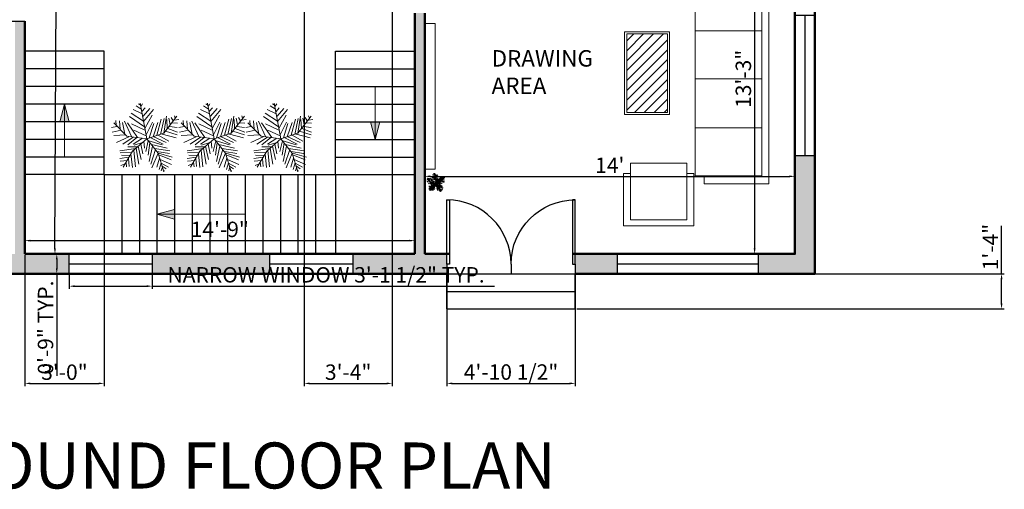
# Model space of a CAD drawing. Units: inches. Extents: x 1647 to 2354, y 1705 to 2321.
# Tile 2 of 4: x 1907 to 2354, y 1705 to 1919. Entities that reach past the tile are written whole.
import ezdxf

# ---------------------------------------------------------------- set-up
doc = ezdxf.new("R2010")
doc.units = ezdxf.units.IN
for name, color, linetype, lineweight in [('A-ANNO-DIMS', 130, 'Continuous', 18), ('A-ANNO-SYMB', 50, 'Continuous', 18), ('A-ANNO-TEXT', 7, 'Continuous', 35), ('A-AREA-IDEN', 7, 'Continuous', 25), ('A-FURN-PATT', 52, 'Continuous', 13), ('A-WALL-PATT', 84, 'Continuous', 13), ('door', 142, 'Continuous', 25), ('fur', 52, 'Continuous', 18), ('stair', 50, 'Continuous', 25), ('tree', 92, 'Continuous', 13), ('wall', 84, 'Continuous', 50), ('window', 242, 'Continuous', 25)]:
    doc.layers.add(name, color=color, linetype=linetype, lineweight=lineweight)
doc.styles.get("Standard").update_dxf_attribs({"font": 'arial.ttf'})
doc.dimstyles.new('ISO-25', dxfattribs={"dimtxt": 7, "dimasz": 2.5, "dimexe": 1.25, "dimexo": 0.625, "dimtad": 1, "dimdec": 0, "dimlunit": 4, "dimtxsty": 'Standard', "dimcen": 2.5, "dimadec": 0, "dimazin": 0, "dimtfac": 1, "dimtdec": 0, "dimtmove": 0, "dimatfit": 3, "dimfxl": 1, "dimarcsym": 0})

# ---------------------------------------------------------------- blocks, each defined once
blk = doc.blocks.new('*U2')
for p, q in [((0, 0), (0, -6)), ((40, 0), (40, -6))]:
    blk.add_line(p, q)
blk.add_lwpolyline([(0, 0), (0, 40), (1.75, 40), (1.75, 0)], close=True)
blk.add_arc((0, 0), 40, 0, 90)
blk = doc.blocks.new('*U6')
for p, q in [((-8.737, 47.138), (-17.069, 52.711)), ((-10.186, 53.64), (-13.084, 55.962)), ((0, 0), (-10.5, 57)), ((-9.099, 51.782), (-6.563, 55.962)), ((-7.65, 43.423), (-2.578, 49.46)), ((-5.839, 35.992), (4.667, 48.067)), ((-3.665, 19.273), (-27.574, 35.527)), ((-5.114, 28.097), (-24.676, 40.636)), ((-7.288, 39.707), (-21.778, 46.673)), ((-5.114, 27.632), (10.463, 46.673)), ((-2.941, 16.486), (8.652, 37.85)), ((16.259, 5.805), (23.142, 31.348)), ((22.055, 7.198), (27.489, 32.277)), ((27, 9), (48, 36)), ((27.127, 9.056), (31.112, 35.992)), ((35.096, 32.741), (37.27, 22.524)), ((38.719, 34.134), (41.979, 28.561)), ((44.153, 36.456), (45.239, 32.741)), ((-47.498, 19.737), (-55.83, 18.344)), ((-31.5, 4.5), (-52.5, 25.5)), ((-48.585, 21.131), (-49.309, 29.026)), ((-43.513, 28.561), (-42.427, 15.558)), ((-38.442, 26.239), (-34.819, 7.663)), ((-35.544, 28.097), (-24.314, 3.947)), ((-14.533, 2.09), (-30.834, 25.31)), ((-24.314, 23.917), (-2.941, 13.7)), ((-1.129, 6.734), (9.014, 26.704)), ((3.942, 1.625), (11.187, 24.381)), ((10.101, 3.483), (17.708, 26.239)), ((31.836, 30.883), (32.561, 16.486)), ((33.285, 16.486), (48.862, 10.913)), ((36.183, 19.737), (48.137, 17.88)), ((40.53, 25.775), (48.862, 24.846)), ((43.791, 29.954), (51.036, 30.883)), ((-40.615, 13.7), (-55.105, 10.913)), ((-33.37, 6.269), (-52.207, 5.34)), ((-28.299, 3.483), (-47.86, -5.805)), ((-21.416, 3.018), (-38.079, -8.128)), ((0, 0), (-31.5, 4.5)), ((-15.982, 2.09), (-30.11, -9.521)), ((0, 0), (-22.5, -19.5)), ((-6.563, 1.161), (-21.416, -8.128)), ((-20.691, 13.7), (-1.129, 4.876)), ((0, 0), (27, 9)), ((0, 0), (18, -22.5)), ((6.478, 1.625), (26.04, -8.592)), ((11.187, 3.483), (30.749, -5.805)), ((18.07, 5.805), (35.096, -3.483)), ((24.229, 7.663), (46.688, 1.625)), ((29.662, 12.307), (48.137, 6.269)), ((-17.431, -15.094), (-42.789, -18.809)), ((-15.257, -12.772), (-30.11, -12.772)), ((-6.563, -5.805), (-19.967, -9.985)), ((-17.069, -15.094), (-12.721, -40.172)), ((-13.446, -11.378), (-8.737, -32.741)), ((-9.461, -8.592), (-6.201, -23.453)), ((-4.752, -3.483), (-3.665, -14.629)), ((2.493, -3.019), (-1.491, -20.202)), ((1.769, -2.555), (24.229, -9.521)), ((5.029, -6.27), (2.131, -25.775)), ((9.014, -11.378), (3.58, -35.992)), ((7.565, -9.056), (32.198, -14.629)), ((12.274, -15.094), (36.907, -18.809)), ((-28.299, -29.026), (-42.789, -31.348)), ((-24.314, -21.596), (-42.427, -22.06)), ((-26.849, -26.24), (-40.253, -25.775)), ((-22.5, -19.5), (-37.5, -45)), ((-29.023, -30.884), (-27.936, -43.887)), ((-25.038, -23.918), (-22.865, -45.281)), ((-20.691, -18.345), (-17.793, -44.352)), ((14.085, -16.951), (6.478, -40.172)), ((18.07, -22.524), (8.289, -45.745)), ((20.244, -30.419), (15.897, -44.816)), ((16.259, -19.738), (36.183, -22.989)), ((18, -22.5), (27, -52.5)), ((18.433, -22.524), (40.53, -29.026)), ((19.157, -25.311), (38.719, -33.206)), ((-30.834, -34.135), (-42.427, -35.528)), ((-34.457, -39.708), (-40.978, -42.494)), ((-32.646, -36.921), (-31.921, -44.352)), ((22.78, -37.85), (19.519, -48.532)), ((21.331, -32.741), (39.081, -40.636)), ((22.78, -38.314), (34.372, -44.816)), ((24.591, -45.745), (23.142, -50.854)), ((24.591, -43.423), (30.749, -47.603)), ((26.764, -49.925), (28.213, -50.854))]:
    blk.add_line(p, q)
blk = doc.blocks.new('*D15')
at = {"layer": 'A-ANNO-DIMS', "color": 0, "lineweight": -2, "transparency": 16777216}
for p, q in [((1909.63, 1812.86), (1909.63, 1819.51)), ((2086.63, 1812.86), (2086.63, 1819.51)), ((1912.13, 1818.26), (2084.13, 1818.26))]:
    blk.add_line(p, q, dxfattribs=at)
at = {"layer": 'A-ANNO-DIMS', "color": 0, "transparency": 16777216}
for points in [[(1912.13, 1818.68), (1912.13, 1817.85), (1909.63, 1818.26)], [(2084.13, 1818.68), (2084.13, 1817.85), (2086.63, 1818.26)]]:
    blk.add_solid(points, dxfattribs=at)
at = {"layer": 'Defpoints', "color": 0, "transparency": 16777216}
for p in [(2086.63, 1818.26), (1909.63, 1812.23), (2086.63, 1812.23)]:
    blk.add_point(p, dxfattribs=at)
at = {"layer": 'A-ANNO-DIMS', "color": 0, "transparency": 16777216, "insert": (1998.13, 1822.46), "char_height": 7, "attachment_point": 5}
blk.add_mtext('14\'-9"', dxfattribs=at)
blk = doc.blocks.new('*D16')
at = {"layer": 'A-ANNO-DIMS', "color": 0, "lineweight": -2, "transparency": 16777216}
for p, q in [((1911.55, 2059.73), (1925.86, 2059.66)), ((1923.34, 1814.66), (1924.6, 2057.16)), ((1910.26, 1812.23), (1924.57, 1812.16))]:
    blk.add_line(p, q, dxfattribs=at)
at = {"layer": 'A-ANNO-DIMS', "color": 0, "transparency": 16777216}
for points in [[(1924.18, 2057.16), (1925.01, 2057.16), (1924.61, 2059.66)], [(1922.92, 1814.66), (1923.75, 1814.66), (1923.32, 1812.16)]]:
    blk.add_solid(points, dxfattribs=at)
at = {"layer": 'Defpoints', "color": 0, "transparency": 16777216}
for p in [(1910.92, 2059.73), (1924.61, 2059.66), (1909.63, 1812.23)]:
    blk.add_point(p, dxfattribs=at)
at = {"layer": 'A-ANNO-DIMS', "color": 0, "transparency": 16777216, "insert": (1919.77, 1935.93), "char_height": 7, "attachment_point": 5, "rotation": 89.702}
blk.add_mtext('20\'-8"', dxfattribs=at)
blk = doc.blocks.new('*D17')
at = {"layer": 'A-ANNO-DIMS', "color": 0, "lineweight": -2, "transparency": 16777216}
for p, q in [((2091.13, 1812.86), (2091.13, 1848.7)), ((2093.63, 1847.45), (2256.63, 1847.45)), ((2259.13, 1812.86), (2259.13, 1848.7))]:
    blk.add_line(p, q, dxfattribs=at)
at = {"layer": 'A-ANNO-DIMS', "color": 0, "transparency": 16777216}
for points in [[(2093.63, 1847.87), (2093.63, 1847.04), (2091.13, 1847.45)], [(2256.63, 1847.87), (2256.63, 1847.04), (2259.13, 1847.45)]]:
    blk.add_solid(points, dxfattribs=at)
at = {"layer": 'Defpoints', "color": 0, "transparency": 16777216}
for p in [(2259.13, 1847.45), (2091.13, 1812.23), (2259.13, 1812.23)]:
    blk.add_point(p, dxfattribs=at)
at = {"layer": 'A-ANNO-DIMS', "color": 0, "transparency": 16777216, "insert": (2175.13, 1851.59), "char_height": 7, "attachment_point": 5}
blk.add_mtext("14'", dxfattribs=at)
blk = doc.blocks.new('*D18')
at = {"layer": 'A-ANNO-DIMS', "color": 0, "lineweight": -2, "transparency": 16777216}
for p, q in [((2258.51, 1971.23), (2239.61, 1971.23)), ((2240.86, 1968.73), (2240.86, 1814.73)), ((2258.51, 1812.23), (2239.61, 1812.23))]:
    blk.add_line(p, q, dxfattribs=at)
at = {"layer": 'A-ANNO-DIMS', "color": 0, "transparency": 16777216}
for points in [[(2240.44, 1968.73), (2241.28, 1968.73), (2240.86, 1971.23)], [(2240.44, 1814.73), (2241.28, 1814.73), (2240.86, 1812.23)]]:
    blk.add_solid(points, dxfattribs=at)
at = {"layer": 'Defpoints', "color": 0, "transparency": 16777216}
for p in [(2259.13, 1971.23), (2240.86, 1812.23), (2259.13, 1812.23)]:
    blk.add_point(p, dxfattribs=at)
at = {"layer": 'A-ANNO-DIMS', "color": 0, "transparency": 16777216, "insert": (2236.66, 1891.73), "char_height": 7, "attachment_point": 5, "rotation": 90}
blk.add_mtext('13\'-3"', dxfattribs=at)
blk = doc.blocks.new('WIN-WIDE-9IN-WALL')
blk.add_line((0, 4.5), (63.83, 4.5))
blk.add_lwpolyline([(0, 9), (63.83, 9), (63.83, 0), (0, 0)], close=True)
blk = doc.blocks.new('WIN-NARROW-9IN-WALL')
blk.add_line((4.5, 0), (4.5, 37.68))
blk.add_lwpolyline([(0, 37.68), (9, 37.68), (9, 0), (0, 0)], close=True)
blk = doc.blocks.new('*D37')
at = {"layer": 'A-ANNO-DIMS', "color": 0, "lineweight": -2, "transparency": 16777216}
for p, q in [((1929.8, 1802.61), (1929.8, 1796.33)), ((1967.48, 1802.61), (1967.48, 1796.33)), ((1932.3, 1797.58), (1964.98, 1797.58)), ((1967.48, 1797.58), (2122.76, 1797.58))]:
    blk.add_line(p, q, dxfattribs=at)
at = {"layer": 'A-ANNO-DIMS', "color": 0, "transparency": 16777216}
for points in [[(1932.3, 1798), (1932.3, 1797.16), (1929.8, 1797.58)], [(1964.98, 1798), (1964.98, 1797.16), (1967.48, 1797.58)]]:
    blk.add_solid(points, dxfattribs=at)
at = {"layer": 'Defpoints', "color": 0, "transparency": 16777216}
for p in [(1929.8, 1803.23), (1967.48, 1803.23), (1967.48, 1797.58)]:
    blk.add_point(p, dxfattribs=at)
at = {"layer": 'A-ANNO-DIMS', "color": 0, "transparency": 16777216, "insert": (2046.37, 1801.83), "char_height": 7, "attachment_point": 5}
blk.add_mtext('NARROW WINDOW 3\'-1 1/2" TYP.', dxfattribs=at)
blk = doc.blocks.new('*D38')
at = {"layer": 'A-ANNO-DIMS', "color": 0, "lineweight": -2, "transparency": 16777216}
for p, q in [((1929.18, 1812.23), (1922.9, 1812.23)), ((1924.15, 1809.73), (1924.15, 1805.73)), ((1929.18, 1803.23), (1922.9, 1803.23)), ((1924.15, 1803.23), (1924.15, 1756.81))]:
    blk.add_line(p, q, dxfattribs=at)
at = {"layer": 'A-ANNO-DIMS', "color": 0, "transparency": 16777216}
for points in [[(1923.74, 1809.73), (1924.57, 1809.73), (1924.15, 1812.23)], [(1923.74, 1805.73), (1924.57, 1805.73), (1924.15, 1803.23)]]:
    blk.add_solid(points, dxfattribs=at)
at = {"layer": 'Defpoints', "color": 0, "transparency": 16777216}
for p in [(1929.8, 1812.23), (1924.15, 1803.23), (1929.8, 1803.23)]:
    blk.add_point(p, dxfattribs=at)
at = {"layer": 'A-ANNO-DIMS', "color": 0, "transparency": 16777216, "insert": (1919.95, 1778.77), "char_height": 7, "attachment_point": 5, "rotation": 90}
blk.add_mtext('0\'-9" TYP.', dxfattribs=at)
blk = doc.blocks.new('*D53')
at = {"layer": 'A-ANNO-DIMS', "color": 0, "lineweight": -2, "transparency": 16777216}
for p, q in [((2101.16, 1802.61), (2101.16, 1752.18)), ((2159.48, 1802.61), (2159.48, 1752.18)), ((2103.66, 1753.43), (2156.98, 1753.43))]:
    blk.add_line(p, q, dxfattribs=at)
at = {"layer": 'A-ANNO-DIMS', "color": 0, "transparency": 16777216}
for points in [[(2103.66, 1753.85), (2103.66, 1753.02), (2101.16, 1753.43)], [(2156.98, 1753.85), (2156.98, 1753.02), (2159.48, 1753.43)]]:
    blk.add_solid(points, dxfattribs=at)
at = {"layer": 'Defpoints', "color": 0, "transparency": 16777216}
for p in [(2101.16, 1803.23), (2159.48, 1803.23), (2159.48, 1753.43)]:
    blk.add_point(p, dxfattribs=at)
at = {"layer": 'A-ANNO-DIMS', "color": 0, "transparency": 16777216, "insert": (2130.32, 1757.68), "char_height": 7, "attachment_point": 5}
blk.add_mtext('4\'-10 1/2"', dxfattribs=at)
blk = doc.blocks.new('*D54')
at = {"layer": 'A-ANNO-DIMS', "color": 0, "lineweight": -2, "transparency": 16777216}
for p, q in [((2352.93, 1803.23), (2352.93, 1824.93)), ((2160.11, 1803.23), (2354.18, 1803.23)), ((2352.93, 1789.73), (2352.93, 1800.73)), ((2160.11, 1787.23), (2354.18, 1787.23))]:
    blk.add_line(p, q, dxfattribs=at)
at = {"layer": 'A-ANNO-DIMS', "color": 0, "transparency": 16777216}
for points in [[(2352.52, 1800.73), (2353.35, 1800.73), (2352.93, 1803.23)], [(2352.52, 1789.73), (2353.35, 1789.73), (2352.93, 1787.23)]]:
    blk.add_solid(points, dxfattribs=at)
at = {"layer": 'Defpoints', "color": 0, "transparency": 16777216}
for p in [(2159.48, 1803.23), (2352.93, 1803.23), (2159.48, 1787.23)]:
    blk.add_point(p, dxfattribs=at)
at = {"layer": 'A-ANNO-DIMS', "color": 0, "transparency": 16777216, "insert": (2348.8, 1815.33), "char_height": 7, "attachment_point": 5, "rotation": 90}
blk.add_mtext('1\'-4"', dxfattribs=at)
blk = doc.blocks.new('*D55')
at = {"layer": 'A-ANNO-DIMS', "color": 0, "lineweight": -2, "transparency": 16777216}
for p, q in [((1909.63, 1811.61), (1909.63, 1752.18)), ((1945.63, 1811.61), (1945.63, 1752.18)), ((1912.13, 1753.43), (1943.13, 1753.43))]:
    blk.add_line(p, q, dxfattribs=at)
at = {"layer": 'A-ANNO-DIMS', "color": 0, "transparency": 16777216}
for points in [[(1912.13, 1753.85), (1912.13, 1753.02), (1909.63, 1753.43)], [(1943.13, 1753.85), (1943.13, 1753.02), (1945.63, 1753.43)]]:
    blk.add_solid(points, dxfattribs=at)
at = {"layer": 'Defpoints', "color": 0, "transparency": 16777216}
for p in [(1909.63, 1812.23), (1945.63, 1812.23), (1945.63, 1753.43)]:
    blk.add_point(p, dxfattribs=at)
at = {"layer": 'A-ANNO-DIMS', "color": 0, "transparency": 16777216, "insert": (1927.63, 1757.63), "char_height": 7, "attachment_point": 5}
blk.add_mtext('3\'-0"', dxfattribs=at)
blk = doc.blocks.new('*D56')
at = {"layer": 'A-ANNO-DIMS', "color": 0, "lineweight": -2, "transparency": 16777216}
for p, q in [((2036.41, 2059.11), (2036.41, 1752.18)), ((2076.41, 2059.11), (2076.41, 1752.18)), ((2038.91, 1753.43), (2073.91, 1753.43))]:
    blk.add_line(p, q, dxfattribs=at)
at = {"layer": 'A-ANNO-DIMS', "color": 0, "transparency": 16777216}
for points in [[(2038.91, 1753.85), (2038.91, 1753.02), (2036.41, 1753.43)], [(2073.91, 1753.85), (2073.91, 1753.02), (2076.41, 1753.43)]]:
    blk.add_solid(points, dxfattribs=at)
at = {"layer": 'Defpoints', "color": 0, "transparency": 16777216}
for p in [(2036.41, 2059.73), (2076.41, 2059.73), (2076.41, 1753.43)]:
    blk.add_point(p, dxfattribs=at)
at = {"layer": 'A-ANNO-DIMS', "color": 0, "transparency": 16777216, "insert": (2056.41, 1757.63), "char_height": 7, "attachment_point": 5}
blk.add_mtext('3\'-4"', dxfattribs=at)

msp = doc.modelspace()

# ---------------------------------------------------------------- hatches: boundary and pattern name
at = {"layer": 'A-ANNO-SYMB'}
h = msp.add_hatch(color=256, dxfattribs=at)
h.dxf.hatch_style = 1
h.paths.add_polyline_path([(1927.63, 1880.23), (1925.48, 1872.23), (1927.63, 1872.23)])
h.paths.add_polyline_path([(1927.63, 1880.23), (1927.63, 1872.23), (1929.78, 1872.23)])
h.paths.add_polyline_path([(1977.63, 1830.23), (1969.63, 1830.23), (1977.63, 1828.08)])
h.paths.add_polyline_path([(1977.63, 1832.38), (1969.63, 1830.23), (1977.63, 1830.23)])
h.paths.add_polyline_path([(2068.63, 1872.23), (2066.48, 1872.23), (2068.63, 1864.23)])
h.paths.add_polyline_path([(2070.78, 1872.23), (2068.63, 1872.23), (2068.63, 1864.23)])
at = {"layer": 'A-FURN-PATT'}
h = msp.add_hatch(dxfattribs=at)
h.set_pattern_fill('ANSI31', color=256)
h.paths.add_polyline_path([(2201.3, 1912.1), (2182.82, 1912.1), (2182.82, 1876.48), (2201.3, 1876.48)])
at = {"layer": 'A-WALL-PATT'}
h = msp.add_hatch(color=256, dxfattribs=at)
h.dxf.hatch_style = 1
h.paths.add_polyline_path([(1737.13, 2214.23), (1778.6, 2214.23), (1778.6, 2223.23), (1728.13, 2223.23), (1728.13, 2080.92), (1737.13, 2080.92)])
h.paths.add_polyline_path([(1785.23, 1812.23), (1737.13, 1812.23), (1737.13, 1856.57), (1728.13, 1856.57), (1728.13, 1803.23), (1785.23, 1803.23)])
h.paths.add_polyline_path([(2020.88, 1812.23), (1967.48, 1812.23), (1967.48, 1803.23), (2020.88, 1803.23)])
h.paths.add_polyline_path([(2101.16, 1807.61), (2101.16, 1812.23), (2091.13, 1812.23), (2091.13, 1921.55), (2086.63, 1921.55), (2086.63, 1812.23), (2058.56, 1812.23), (2058.56, 1803.23), (2101.16, 1803.23)])
h.paths.add_polyline_path([(1929.8, 1812.23), (1909.63, 1812.23), (1909.63, 1848.23), (1909.63, 1917.89), (1905.13, 1917.89), (1905.13, 1812.23), (1882.72, 1812.23), (1849.06, 1812.23), (1849.06, 1803.23), (1929.8, 1803.23)])
h.paths.add_polyline_path([(2178.59, 1812.23), (2159.48, 1812.23), (2159.48, 1807.61), (2159.48, 1803.23), (2178.59, 1803.23)])
h.paths.add_polyline_path([(2268.13, 1856.83), (2259.13, 1856.83), (2259.13, 1815.23), (2259.13, 1812.23), (2242.42, 1812.23), (2242.42, 1803.23), (2268.13, 1803.23)])

# ---------------------------------------------------------------- linework, layer by layer
at = {"layer": 'A-ANNO-SYMB'}
for p, q in [((2068.63, 1888.23), (2068.63, 1864.23)), ((1927.63, 1880.23), (1925.48, 1872.23)), ((1927.63, 1856.23), (1927.63, 1880.23)), ((1927.63, 1880.23), (1929.78, 1872.23)), ((2068.63, 1864.23), (2066.48, 1872.23)), ((2068.63, 1864.23), (2070.78, 1872.23)), ((1969.63, 1830.23), (1977.63, 1832.38)), ((2009.63, 1830.23), (1969.63, 1830.23)), ((1969.63, 1830.23), (1977.63, 1828.08))]:
    msp.add_line(p, q, dxfattribs=at)
at = {"layer": 'fur'}
for p, q in [((2247.32, 1938.45), (2247.32, 1844.07)), ((2213.66, 1913.56), (2243.99, 1913.56)), ((2213.93, 1891.76), (2244.26, 1891.76)), ((2213.88, 1869.52), (2244.21, 1869.52)), ((2184.61, 1848.77), (2181.31, 1848.77)), ((2181.31, 1848.77), (2181.31, 1824.98)), ((2184.61, 1848.77), (2184.61, 1848.77)), ((2213.35, 1848.77), (2210.14, 1848.77)), ((2213.35, 1824.98), (2213.35, 1848.77)), ((2217.9, 1844.07), (2217.9, 1847.66)), ((2247.32, 1844.07), (2217.9, 1844.07)), ((2181.31, 1824.98), (2213.35, 1824.98))]:
    msp.add_line(p, q, dxfattribs=at)
for points in [[(2244.21, 1934.94), (2213.88, 1934.94), (2213.88, 1847.66), (2244.21, 1847.66)], [(2091.13, 1916.87), (2095.96, 1916.87), (2095.96, 1850.72), (2091.13, 1850.72)], [(2202.3, 1913.1), (2181.82, 1913.1), (2181.82, 1875.48), (2202.3, 1875.48)], [(2201.3, 1912.1), (2182.82, 1912.1), (2182.82, 1876.48), (2201.3, 1876.48)], [(2184.61, 1853.5), (2210.14, 1853.5), (2210.14, 1827.72), (2184.61, 1827.72)]]:
    msp.add_lwpolyline(points, close=True, dxfattribs=at)
at = {"layer": 'stair'}
for p, q in [((1945.63, 1904.23), (1909.63, 1904.23)), ((1945.63, 1848.23), (1945.63, 1904.23)), ((2050.63, 1848.23), (2050.63, 1904.23)), ((2050.63, 1904.23), (2086.63, 1904.23)), ((1945.63, 1896.23), (1909.63, 1896.23)), ((2050.63, 1896.23), (2086.63, 1896.23)), ((1945.63, 1888.23), (1909.63, 1888.23)), ((2050.63, 1888.23), (2086.63, 1888.23)), ((1945.63, 1880.23), (1909.63, 1880.23)), ((2050.63, 1880.23), (2086.63, 1880.23)), ((1945.63, 1872.23), (1909.63, 1872.23)), ((2050.63, 1872.23), (2086.63, 1872.23)), ((1945.63, 1864.23), (1909.63, 1864.23)), ((2050.63, 1864.23), (2086.63, 1864.23)), ((1945.63, 1856.23), (1909.63, 1856.23)), ((2050.63, 1856.23), (2086.63, 1856.23)), ((1909.63, 1812.23), (1909.63, 1848.23)), ((1945.63, 1848.23), (1909.63, 1848.23)), ((1945.63, 1848.23), (2050.63, 1848.23)), ((1945.63, 1848.23), (1945.63, 1812.23)), ((1953.63, 1848.23), (1953.63, 1812.23)), ((1961.63, 1848.23), (1961.63, 1812.23)), ((1969.63, 1848.23), (1969.63, 1812.23)), ((1977.63, 1848.23), (1977.63, 1812.23)), ((1985.63, 1848.23), (1985.63, 1812.23)), ((1993.63, 1848.23), (1993.63, 1812.23)), ((2001.63, 1848.23), (2001.63, 1812.23)), ((2009.63, 1848.23), (2009.63, 1812.23)), ((2017.63, 1848.23), (2017.63, 1812.23)), ((2025.63, 1848.23), (2025.63, 1812.23)), ((2033.63, 1848.23), (2033.63, 1812.23)), ((2041.63, 1848.23), (2041.63, 1812.23)), ((2050.63, 1848.23), (2086.63, 1848.23)), ((2050.63, 1848.23), (2050.63, 1812.23)), ((2101.16, 1803.23), (2159.48, 1803.23)), ((2101.16, 1787.23), (2101.16, 1803.23)), ((2159.48, 1787.23), (2159.48, 1803.23)), ((2101.16, 1795.23), (2159.48, 1795.23)), ((2101.16, 1787.23), (2159.48, 1787.23))]:
    msp.add_line(p, q, dxfattribs=at)
at = {"layer": 'wall'}
for p, q in [((2268.13, 2223.23), (2268.13, 1803.23)), ((2259.13, 1971.23), (2259.13, 1815.23)), ((2086.63, 1812.23), (2086.63, 1921.55)), ((2091.13, 1812.23), (2091.13, 1921.55)), ((1909.63, 1917.89), (1909.63, 1812.23)), ((1909.63, 1812.23), (1929.8, 1812.23)), ((1909.63, 1812.23), (1929.8, 1812.23)), ((2086.63, 1812.23), (2058.56, 1812.23)), ((2102.44, 1812.23), (2091.13, 1812.23)), ((2259.13, 1812.23), (2158.21, 1812.23)), ((2101.16, 1803.23), (1728.13, 1803.23)), ((2268.13, 1803.23), (2159.48, 1803.23))]:
    msp.add_line(p, q, dxfattribs=at)
for points in [[(2101.16, 1803.23), (1728.13, 1803.23), (1728.13, 2223.23), (2268.13, 2223.23), (2268.13, 1803.23), (2159.48, 1803.23)], [(2259.13, 1971.23), (2259.13, 1812.23), (2158.21, 1812.23)], [(2086.63, 1812.23), (1909.63, 1812.23)], [(2102.44, 1812.23), (2091.13, 1812.23)]]:
    msp.add_lwpolyline(points, dxfattribs=at)

# ---------------------------------------------------------------- block references
at = {"layer": 'door', "xscale": -1, "rotation": 90}
msp.add_blockref('*U2', (1903.63, 1957.89), dxfattribs=at)
at = {"layer": 'door', "yscale": 0.7290180259199005, "zscale": 0.7290180259199005}
for p, xscale in [((2101.16, 1807.61), 0.7290180259199005), ((2159.48, 1807.61), -0.7290180259199005)]:
    msp.add_blockref('*U2', p, dxfattribs=dict(at, xscale=xscale))
at = {"layer": 'tree'}
for p, xscale, yscale, zscale in [((1964.99, 1864.45), 0.2858091163346259, 0.2858091163346259, 0.2858091163346259), ((1995.56, 1864.45), 0.2858091163346259, 0.2858091163346259, 0.2858091163346259), ((2025.85, 1864.45), 0.2858091163346259, 0.2858091163346259, 0.2858091163346259), ((2096.34, 1844.48), 0.0769272842129196, 0.0769272842129196, 0.0769272842129196)]:
    msp.add_blockref('*U6', p, dxfattribs=dict(at, xscale=xscale, yscale=yscale, zscale=zscale))
at = {"layer": 'window'}
for name, p, rotation in [('WIN-WIDE-9IN-WALL', (2259.13, 1920.66), 270.0000000000003), ('WIN-NARROW-9IN-WALL', (1929.8, 1812.23), 269.9999999999994), ('WIN-NARROW-9IN-WALL', (2020.88, 1812.23), 269.999999999999)]:
    msp.add_blockref(name, p, dxfattribs=dict(at, rotation=rotation))
msp.add_blockref('WIN-WIDE-9IN-WALL', (2178.59, 1803.23), dxfattribs=at)

# ---------------------------------------------------------------- texts
at = {"layer": 'A-ANNO-TEXT', "insert": (1855.17, 1726.6), "char_height": 20.8881, "attachment_point": 1}
msp.add_mtext_dynamic_manual_height_columns('GROUND FLOOR PLAN', width=3558.7841, gutter_width=104.44, heights=[0], dxfattribs=at)
at = {"layer": 'A-AREA-IDEN', "insert": (2121.5, 1904.76), "char_height": 7.465, "attachment_point": 1}
msp.add_mtext_dynamic_manual_height_columns('DRAWING\\PAREA', width=263.8302, gutter_width=37.32, heights=[0], dxfattribs=at)

# ---------------------------------------------------------------- dimensions: what is measured, and where the dimension line sits
at = {"layer": 'A-ANNO-DIMS'}
dim = msp.add_aligned_dim(p1=(1909.63, 1812.23), p2=(1910.92, 2059.73), distance=-13.69, dimstyle='ISO-25', override={"dimclrd": 0, "dimclre": 0, "dimclrt": 0}, dxfattribs=at)
dim.commit()
dim.dimension.update_dxf_attribs({"geometry": '*D16', "text_midpoint": (1919.77, 1935.93)})
for base, p1, p2, override, picture, middle in [((2076.41, 1753.43), (2036.41, 2059.73), (2076.41, 2059.73), {"dimdec": 1, "dimlfac": 1, "dimrnd": 0, "dimzin": 1, "dimdsep": 46, "dimlunit": 4, "dimfrac": 2}, '*D56', (2056.41, 1757.63)), ((2259.13, 1847.45), (2091.13, 1812.23), (2259.13, 1812.23), {"dimclrd": 0, "dimclre": 0, "dimclrt": 0}, '*D17', (2175.13, 1851.59)), ((2086.63, 1818.26), (1909.63, 1812.23), (2086.63, 1812.23), {"dimclrd": 0, "dimclre": 0, "dimclrt": 0}, '*D15', (1998.13, 1822.46)), ((1945.63, 1753.43), (1909.63, 1812.23), (1945.63, 1812.23), {"dimdec": 1, "dimlfac": 1, "dimrnd": 0, "dimzin": 1, "dimdsep": 46, "dimlunit": 4, "dimfrac": 2}, '*D55', (1927.63, 1757.63)), ((2159.48, 1753.43), (2101.16, 1803.23), (2159.48, 1803.23), {"dimdec": 1, "dimlfac": 1, "dimrnd": 0, "dimzin": 1, "dimdsep": 46, "dimlunit": 4, "dimfrac": 2}, '*D53', (2130.32, 1757.68))]:
    dim = msp.add_linear_dim(base=base, p1=p1, p2=p2, dimstyle='ISO-25', override=override, dxfattribs=at)
    dim.commit()
    dim.dimension.update_dxf_attribs({"geometry": picture, "text_midpoint": middle})
for base, p1, p2, override, picture, middle in [((2240.86, 1812.23), (2259.13, 1971.23), (2259.13, 1812.23), {"dimclrd": 0, "dimclre": 0, "dimclrt": 0}, '*D18', (2236.66, 1891.73)), ((2352.93, 1803.23), (2159.48, 1787.23), (2159.48, 1803.23), {"dimdec": 1, "dimlfac": 1, "dimrnd": 0, "dimzin": 1, "dimdsep": 46, "dimlunit": 4, "dimfrac": 2}, '*D54', (2348.8, 1815.33))]:
    dim = msp.add_linear_dim(base=base, p1=p1, p2=p2, angle=90, dimstyle='ISO-25', override=override, dxfattribs=at)
    dim.commit()
    dim.dimension.update_dxf_attribs({"geometry": picture, "text_midpoint": middle})
dim = msp.add_linear_dim(base=(1967.48, 1797.58), p1=(1929.8, 1803.23), p2=(1967.48, 1803.23), text='NARROW WINDOW <> TYP.', dimstyle='ISO-25', override={"dimdec": 1, "dimlfac": 1, "dimrnd": 0, "dimzin": 1, "dimdsep": 46, "dimlunit": 4, "dimfrac": 2}, dxfattribs=at)
dim.commit()
dim.dimension.update_dxf_attribs({"geometry": '*D37', "text_midpoint": (2046.37, 1801.83)})
dim = msp.add_linear_dim(base=(1924.15, 1803.23), p1=(1929.8, 1812.23), p2=(1929.8, 1803.23), angle=270, text='<> TYP.', dimstyle='ISO-25', override={"dimdec": 1, "dimlfac": 1, "dimrnd": 0, "dimzin": 1, "dimdsep": 46, "dimlunit": 4, "dimfrac": 2}, dxfattribs=at)
dim.commit()
dim.dimension.update_dxf_attribs({"geometry": '*D38', "text_midpoint": (1919.95, 1778.77)})

doc.saveas('drawing.dxf')
